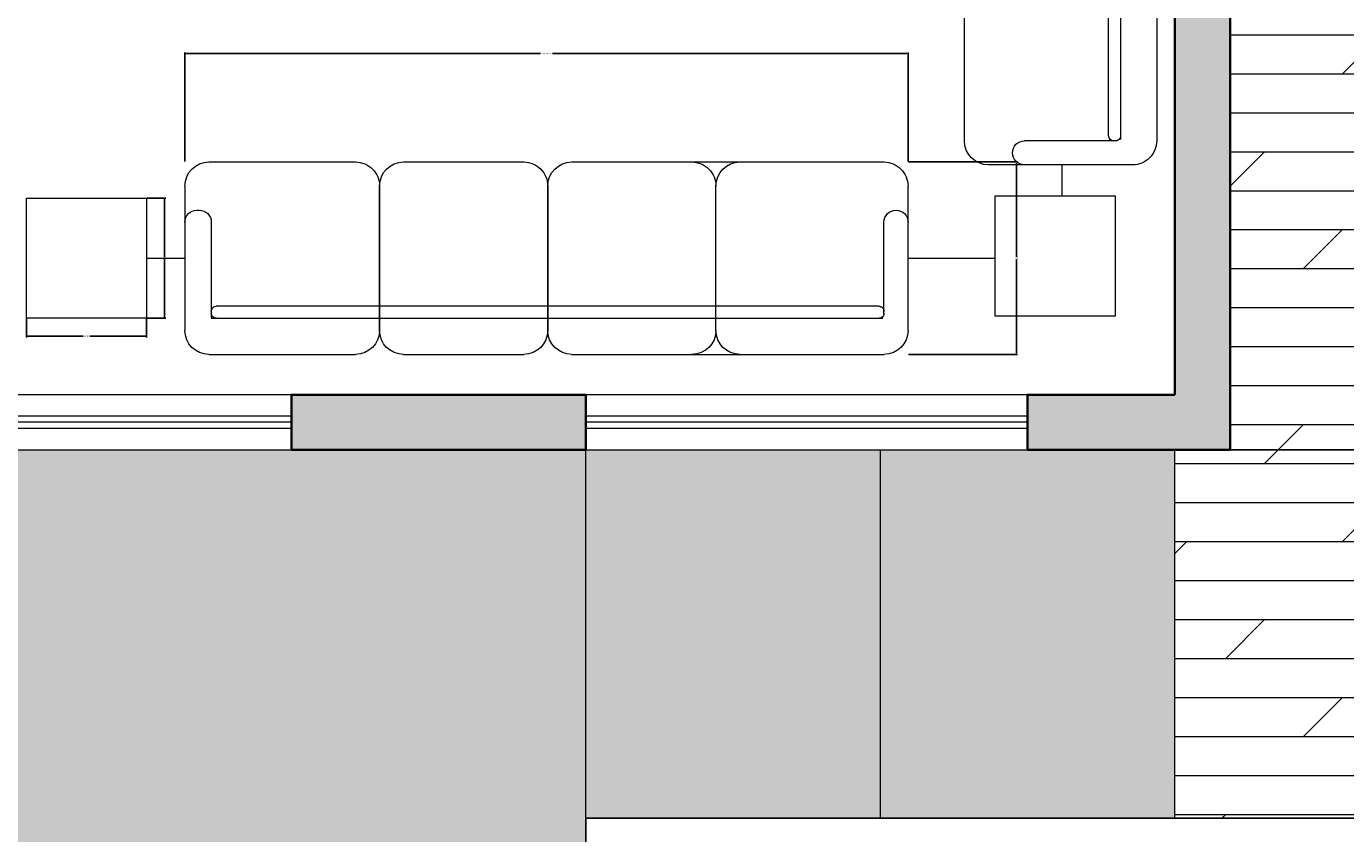
# Model space of a CAD drawing. Units: inches. Extents: x 84 to 1044, y -280 to 906.
# Tile 40 of 105: x 700 to 915, y 29 to 160. Entities that reach past the tile are written whole.
import ezdxf

# ---------------------------------------------------------------- set-up
doc = ezdxf.new("R2010")
doc.units = ezdxf.units.IN
for name, color, linetype, lineweight in [('A-ANNO-DIMS', 2, 'Continuous', 18), ('A-FURN', 8, 'Continuous', 15), ('L-HRDS', 32, 'Continuous', 18), ('L-POOL', 151, 'Continuous', 25), ('WALL', 250, 'Continuous', 35), ('WINDOW', 160, 'Continuous', 13)]:
    doc.layers.add(name, color=color, linetype=linetype, lineweight=lineweight)
for name, color, linetype, lineweight, true_color in [('A-FLOR-PATT', 251, 'Continuous', 9, 0x705861), ('A-WALL-PATT', 251, 'Continuous', 9, 0x636466), ('L-HRDS-PATT', 23, 'Continuous', 9, 0xc2877b), ('L-PLNT-PATT', 9, 'Continuous', 9, 0xafd9aa)]:
    doc.layers.add(name, color=color, linetype=linetype, lineweight=lineweight, true_color=true_color)
doc.styles.get("Standard").update_dxf_attribs({"font": 'arial.ttf'})
doc.dimstyles.get("Standard").update_dxf_attribs({"dimtxt": 0.18, "dimasz": 0.18, "dimexe": 0.18, "dimexo": 0.0625, "dimgap": 0.09, "dimtad": 0, "dimtih": 1, "dimtoh": 1, "dimdec": 4, "dimzin": 0, "dimdsep": 46, "dimtxsty": 'Standard', "dimcen": 0.09, "dimadec": 0, "dimazin": 0, "dimtfac": 1, "dimtdec": 4, "dimtofl": 0, "dimtmove": 0, "dimatfit": 3, "dimfxl": 1, "dimtolj": 1, "dimtzin": 0, "dimarcsym": 0})

# ---------------------------------------------------------------- blocks, each defined once
blk = doc.blocks.new('SOFA-4-SEAT')
for p, q in [((3.92, 31.33), (27.81, 31.33)), ((27.81, 31.33), (27.81, 31.33)), ((35.65, 31.33), (55.23, 31.33)), ((55.23, 31.33), (55.23, 31.33)), ((63.07, 31.33), (113.96, 31.33)), ((113.96, 31.33), (113.96, 31.33)), ((0, 3.91), (0, 27.42)), ((31.73, 27.42), (31.73, 3.91)), ((31.73, 3.91), (31.73, 27.42)), ((59.15, 3.91), (59.15, 27.42)), ((59.15, 27.42), (59.15, 3.91)), ((86.57, 27.42), (86.57, 3.91)), ((117.88, 27.42), (117.88, 3.91)), ((4.31, 12.82), (4.31, 25.46)), ((4.31, 25.46), (11.69, 25.46)), ((4.31, 24.28), (4.31, 24.67)), ((5.09, 25.46), (11.69, 25.46)), ((11.69, 25.46), (113.76, 25.46)), ((11.69, 25.46), (113.18, 25.46)), ((113.96, 24.67), (113.96, 24.28)), ((113.96, 24.28), (113.96, 9.79)), ((13.66, 23.5), (5.09, 23.5)), ((113.18, 23.5), (13.66, 23.5)), ((4.31, 9.79), (4.31, 12.82)), ((1.96, 7.83), (2.35, 7.83)), ((115.92, 7.83), (115.92, 7.83)), ((27.81, 0), (3.92, 0)), ((27.81, 0), (27.81, 0)), ((55.23, 0), (35.65, 0)), ((55.23, 0), (55.23, 0)), ((113.96, 0), (63.07, 0)), ((113.96, 0), (113.96, 0))]:
    blk.add_line(p, q)
for centre, radius, start, end in [((3.92, 27.42), 3.92, 90, 180), ((27.81, 27.42), 3.92, 0, 90), ((35.65, 27.42), 3.92, 90, 180), ((55.23, 27.42), 3.92, 0, 90), ((63.07, 27.42), 3.92, 90, 180), ((82.65, 27.42), 3.92, 0, 90), ((90.48, 27.42), 3.92, 90, 180), ((113.96, 27.42), 3.92, 0, 90), ((5.09, 24.67), 0.783, 90, 180), ((5.09, 24.28), 0.783, 180, 270), ((113.18, 24.67), 0.783, 0, 90), ((113.18, 24.28), 0.783, 270, 0), ((1.96, 9.79), 1.96, 180, 270), ((2.35, 9.79), 1.96, 270, 0), ((115.92, 9.79), 1.96, 180, 270), ((115.92, 9.79), 1.96, 270, 0), ((3.92, 3.91), 3.92, 180, 270), ((27.81, 3.91), 3.92, 270, 0), ((35.65, 3.91), 3.92, 180, 270), ((55.23, 3.91), 3.92, 270, 0), ((63.07, 3.91), 3.92, 180, 270), ((82.65, 3.91), 3.92, 270, 0), ((90.48, 3.91), 3.92, 180, 270), ((113.96, 3.91), 3.92, 270, 0)]:
    blk.add_arc(centre, radius, start, end)
blk = doc.blocks.new('SOFA-2-SEAT')
for p, q in [((27.42, 63.46), (3.92, 63.46)), ((7.83, 61.5), (7.83, 61.5)), ((0, 59.54), (0, 59.54)), ((0, 59.54), (0, 35.65)), ((24.29, 59.54), (9.79, 59.54)), ((23.5, 58.76), (23.5, 13.66)), ((24.68, 59.54), (24.29, 59.54)), ((25.46, 11.69), (25.46, 59.35)), ((25.46, 11.69), (25.46, 58.76)), ((31.34, 59.54), (31.34, 59.54)), ((31.34, 35.65), (31.34, 59.54)), ((3.92, 31.73), (27.42, 31.73)), ((27.42, 31.73), (3.92, 31.73)), ((0, 27.81), (0, 27.81)), ((0, 27.81), (0, 3.92)), ((31.34, 27.81), (31.34, 27.81)), ((31.34, 3.92), (31.34, 27.81)), ((23.5, 13.66), (23.5, 5.09)), ((25.46, 5.09), (25.46, 11.69)), ((25.46, 4.31), (25.46, 11.69)), ((9.79, 4.31), (12.83, 4.31)), ((12.83, 4.31), (25.46, 4.31)), ((24.29, 4.31), (24.68, 4.31)), ((7.83, 1.96), (7.83, 2.35)), ((3.92, 0), (27.42, 0))]:
    blk.add_line(p, q)
for centre, radius, start, end in [((3.92, 59.54), 3.92, 90, 180), ((9.79, 61.5), 1.96, 90, 180), ((27.42, 59.54), 3.92, 360, 90), ((9.79, 61.5), 1.96, 180, 270), ((24.29, 58.76), 0.783, 90, 180), ((24.68, 58.76), 0.783, 360, 90), ((3.92, 35.65), 3.92, 180, 270), ((27.42, 35.65), 3.92, 270, 360), ((3.92, 27.81), 3.92, 90, 180), ((27.42, 27.81), 3.92, 360, 90), ((9.79, 2.35), 1.96, 90, 180), ((24.29, 5.09), 0.783, 180, 270), ((24.68, 5.09), 0.783, 270, 360), ((3.92, 3.92), 3.92, 180, 270), ((27.42, 3.92), 3.92, 270, 360), ((9.79, 1.96), 1.96, 180, 270)]:
    blk.add_arc(centre, radius, start, end)
blk = doc.blocks.new('TABLE-END-SQUARE')
for p, q in [((0, 0), (0, 19.59)), ((0, 19.59), (19.58, 19.59)), ((19.58, 19.59), (19.58, 0)), ((19.58, 0), (0, 0))]:
    blk.add_line(p, q)
blk = doc.blocks.new('WIN-72IN')
for p, q in [((72, 9), (0, 9)), ((72, 5.5), (0, 5.5)), ((72, 4.5), (0, 4.5)), ((72, 3.5), (0, 3.5)), ((0, 0), (72, 0))]:
    blk.add_line(p, q)
blk = doc.blocks.new('*D52')
at = {"layer": 'A-ANNO-DIMS', "color": 0, "lineweight": -2, "transparency": 16777216}
for p, q in [((725.7, 138.09), (725.7, 155.89)), ((725.88, 155.71), (783.66, 155.71)), ((843.4, 155.71), (785.61, 155.71)), ((843.58, 138.09), (843.58, 155.89))]:
    blk.add_line(p, q, dxfattribs=at)
at = {"layer": 'A-ANNO-DIMS', "color": 0, "transparency": 16777216}
for points in [[(725.88, 155.74), (725.88, 155.68), (725.7, 155.71)], [(843.4, 155.74), (843.4, 155.68), (843.58, 155.71)]]:
    blk.add_solid(points, dxfattribs=at)
at = {"layer": 'Defpoints', "color": 0, "transparency": 16777216}
for p in [(843.58, 155.71), (725.7, 138.03), (843.58, 138.03)]:
    blk.add_point(p, dxfattribs=at)
at = {"layer": 'A-ANNO-DIMS', "color": 0, "transparency": 16777216, "insert": (784.64, 155.71), "char_height": 0.18, "attachment_point": 5}
blk.add_mtext('\\A1;SOFA 118 TYP.', dxfattribs=at)
blk = doc.blocks.new('*D53')
at = {"layer": 'A-ANNO-DIMS', "color": 0, "lineweight": -2, "transparency": 16777216}
for p, q in [((843.64, 138.03), (861.44, 138.03)), ((861.26, 137.85), (861.26, 122.54)), ((861.26, 106.87), (861.26, 122.18)), ((843.64, 106.69), (861.44, 106.69))]:
    blk.add_line(p, q, dxfattribs=at)
at = {"layer": 'A-ANNO-DIMS', "color": 0, "transparency": 16777216}
for points in [[(861.23, 137.85), (861.29, 137.85), (861.26, 138.03)], [(861.23, 106.87), (861.29, 106.87), (861.26, 106.69)]]:
    blk.add_solid(points, dxfattribs=at)
at = {"layer": 'Defpoints', "color": 0, "transparency": 16777216}
for p in [(843.58, 138.03), (843.58, 106.69), (861.26, 106.69)]:
    blk.add_point(p, dxfattribs=at)
at = {"layer": 'A-ANNO-DIMS', "color": 0, "transparency": 16777216, "insert": (861.26, 122.36), "char_height": 0.18, "attachment_point": 5}
blk.add_mtext('\\A1;31 TYP.', dxfattribs=at)
blk = doc.blocks.new('*D56')
at = {"layer": 'A-ANNO-DIMS', "color": 0, "lineweight": -2, "transparency": 16777216}
for p, q in [((719.51, 132.15), (722.57, 132.15)), ((722.39, 131.97), (722.39, 122.54)), ((722.39, 112.75), (722.39, 122.18)), ((719.51, 112.57), (722.57, 112.57))]:
    blk.add_line(p, q, dxfattribs=at)
at = {"layer": 'A-ANNO-DIMS', "color": 0, "transparency": 16777216}
for points in [[(722.36, 131.97), (722.42, 131.97), (722.39, 132.15)], [(722.36, 112.75), (722.42, 112.75), (722.39, 112.57)]]:
    blk.add_solid(points, dxfattribs=at)
at = {"layer": 'Defpoints', "color": 0, "transparency": 16777216}
for p in [(719.45, 132.15), (722.39, 132.15), (719.45, 112.57)]:
    blk.add_point(p, dxfattribs=at)
at = {"layer": 'A-ANNO-DIMS', "color": 0, "transparency": 16777216, "insert": (722.39, 122.36), "char_height": 0.18, "attachment_point": 5}
blk.add_mtext('\\A1;END TABLE 20 TYP.', dxfattribs=at)
blk = doc.blocks.new('*D57')
at = {"layer": 'A-ANNO-DIMS', "color": 0, "lineweight": -2, "transparency": 16777216}
for p, q in [((699.86, 112.5), (699.86, 109.45)), ((719.45, 112.5), (719.45, 109.45)), ((700.04, 109.63), (709.13, 109.63)), ((719.27, 109.63), (710.19, 109.63))]:
    blk.add_line(p, q, dxfattribs=at)
at = {"layer": 'A-ANNO-DIMS', "color": 0, "transparency": 16777216}
for points in [[(700.04, 109.66), (700.04, 109.6), (699.86, 109.63)], [(719.27, 109.66), (719.27, 109.6), (719.45, 109.63)]]:
    blk.add_solid(points, dxfattribs=at)
at = {"layer": 'Defpoints', "color": 0, "transparency": 16777216}
for p in [(699.86, 112.57), (719.45, 112.57), (719.45, 109.63)]:
    blk.add_point(p, dxfattribs=at)
at = {"layer": 'A-ANNO-DIMS', "color": 0, "transparency": 16777216, "insert": (709.66, 109.63), "char_height": 0.18, "attachment_point": 5}
blk.add_mtext('\\A1;20 TYP.', dxfattribs=at)
blk = doc.blocks.new('*D63')
at = {"layer": 'A-ANNO-DIMS', "color": 0, "lineweight": -2, "transparency": 16777216}
for p, q in [((833.14, 709.12), (1043.77, 709.12)), ((1043.59, 708.94), (1043.59, 400.3)), ((1043.59, 91.3), (1043.59, 399.94)), ((896.14, 91.12), (1043.77, 91.12))]:
    blk.add_line(p, q, dxfattribs=at)
at = {"layer": 'A-ANNO-DIMS', "color": 0, "transparency": 16777216}
for points in [[(1043.56, 708.94), (1043.62, 708.94), (1043.59, 709.12)], [(1043.56, 91.3), (1043.62, 91.3), (1043.59, 91.12)]]:
    blk.add_solid(points, dxfattribs=at)
at = {"layer": 'Defpoints', "color": 0, "transparency": 16777216}
for p in [(833.07, 709.12), (1043.59, 709.12), (896.07, 91.12)]:
    blk.add_point(p, dxfattribs=at)
at = {"layer": 'A-ANNO-DIMS', "color": 0, "transparency": 16777216, "insert": (1043.59, 400.12), "char_height": 0.18, "attachment_point": 5}
blk.add_mtext('\\A1;618', dxfattribs=at)
blk = doc.blocks.new('*D69')
at = {"layer": 'A-ANNO-DIMS', "color": 0, "lineweight": -2, "transparency": 16777216}
for p, q in [((896.14, 91.12), (1043.77, 91.12)), ((1043.59, 90.94), (1043.59, 61.3)), ((1043.59, 31.3), (1043.59, 60.94)), ((983.14, 31.12), (1043.77, 31.12))]:
    blk.add_line(p, q, dxfattribs=at)
at = {"layer": 'A-ANNO-DIMS', "color": 0, "transparency": 16777216}
for points in [[(1043.56, 90.94), (1043.62, 90.94), (1043.59, 91.12)], [(1043.56, 31.3), (1043.62, 31.3), (1043.59, 31.12)]]:
    blk.add_solid(points, dxfattribs=at)
at = {"layer": 'Defpoints', "color": 0, "transparency": 16777216}
for p in [(896.07, 91.12), (983.07, 31.12), (1043.59, 31.12)]:
    blk.add_point(p, dxfattribs=at)
at = {"layer": 'A-ANNO-DIMS', "color": 0, "transparency": 16777216, "insert": (1043.59, 61.12), "char_height": 0.18, "attachment_point": 5}
blk.add_mtext('\\A1;60', dxfattribs=at)

msp = doc.modelspace()

# ---------------------------------------------------------------- hatches: boundary and pattern name
at = {"layer": 'A-FLOR-PATT', "transparency": 33554597}
h = msp.add_hatch(dxfattribs=at)
h.set_pattern_fill('DOLMIT', color=256)
h.paths.add_polyline_path([(983.074, 265.12), (896.074, 265.12), (896.074, 91.12), (887.074, 91.12), (887.074, 31.12), (983.074, 31.12)])
at = {"layer": 'A-WALL-PATT', "transparency": 33554597}
h = msp.add_hatch(color=256, dxfattribs=at)
h.dxf.hatch_style = 1
h.paths.add_polyline_path([(671.074, 100.12), (647.074, 100.12), (647.074, 160.12), (641.074, 160.12), (620.824, 160.12), (620.824, 151.12), (638.074, 151.12), (638.074, 91.12), (671.074, 91.12)])
h.paths.add_polyline_path([(791.074, 100.12), (743.074, 100.12), (743.074, 91.12), (791.074, 91.12)])
h.paths.add_polyline_path([(896.074, 346.12), (887.074, 346.12), (887.074, 334.12), (870.955, 334.12), (833.074, 334.12), (804.574, 334.12), (804.574, 328.12), (887.074, 328.12), (887.074, 100.12), (863.074, 100.12), (863.074, 91.12), (896.074, 91.12)])
h.paths.add_polyline_path([(507.574, 154.729), (507.574, 160.12), (464.074, 160.12), (464.074, 247.12), (641.074, 247.12), (641.074, 208.12), (647.074, 208.12), (647.074, 328.12), (659.074, 328.12), (659.074, 334.12), (617.074, 334.12), (617.074, 328.12), (641.074, 328.12), (641.074, 256.12), (545.074, 256.12), (545.074, 328.12), (569.074, 328.12), (569.074, 334.12), (518.074, 334.12), (518.074, 325.12), (536.074, 325.12), (536.074, 256.12), (464.074, 256.12), (464.074, 325.12), (482.074, 325.12), (482.074, 334.12), (455.074, 334.12), (455.074, 160.12), (413.127, 160.12), (413.127, 151.12), (455.074, 151.12), (455.074, 91.12), (464.074, 91.12), (464.074, 151.12), (507.574, 151.12)])
h.paths.add_polyline_path([(572.824, 160.12), (555.574, 160.12), (555.574, 151.12), (572.824, 151.12)], flags=17)
h.paths.add_polyline_path([(341.127, 160.12), (299.179, 160.12), (299.179, 211.12), (294.179, 211.12), (290.179, 211.12), (290.179, 151.12), (341.127, 151.12)])
h.paths.add_polyline_path([(299.179, 256.12), (212.179, 256.12), (212.179, 274.12), (203.179, 274.12), (203.179, 247.12), (299.179, 247.12)])
h.paths.add_polyline_path([(212.179, 514.12), (398.074, 514.12), (398.074, 519.12), (398.074, 520.12), (212.179, 520.12), (212.179, 574.12), (203.179, 574.12), (203.179, 310.12), (212.179, 310.12), (212.179, 328.12), (290.179, 328.12), (290.179, 292.12), (299.179, 292.12), (299.179, 328.12), (332.179, 328.12), (332.179, 334.12), (212.179, 334.12)])
h.paths.add_polyline_path([(287.127, 709.12), (203.179, 709.12), (203.179, 646.12), (212.179, 646.12), (212.179, 700.12), (287.127, 700.12)])
h.paths.add_polyline_path([(470.074, 709.12), (359.127, 709.12), (359.127, 700.12), (434.074, 700.12), (434.074, 574.12), (440.074, 574.12), (440.074, 622.12), (464.074, 622.12), (464.074, 628.12), (440.074, 628.12), (440.074, 700.12), (470.074, 700.12)])
h.paths.add_polyline_path([(572.074, 709.12), (506.074, 709.12), (506.074, 700.12), (536.074, 700.12), (536.074, 628.12), (494.074, 628.12), (494.074, 622.12), (536.074, 622.12), (536.074, 520.12), (440.074, 520.12), (440.074, 544.12), (434.074, 544.12), (434.074, 514.12), (644.074, 514.12), (644.074, 519.12), (644.074, 544.12), (638.074, 544.12), (638.074, 520.12), (542.074, 520.12), (542.074, 622.12), (584.074, 622.12), (584.074, 628.12), (542.074, 628.12), (542.074, 700.12), (572.074, 700.12)])
h.paths.add_polyline_path([(698.074, 709.12), (608.074, 709.12), (608.074, 700.12), (638.074, 700.12), (638.074, 628.12), (614.074, 628.12), (614.074, 622.12), (638.074, 622.12), (638.074, 574.12), (644.074, 574.12), (644.074, 700.12), (698.074, 700.12)])
h.paths.add_polyline_path([(833.074, 709.12), (770.074, 709.12), (770.074, 700.12), (824.074, 700.12), (824.074, 646.12), (833.074, 646.12)])
h.paths.add_polyline_path([(833.074, 574.12), (824.074, 574.12), (824.074, 520.12), (791.244, 520.12), (712.904, 520.12), (680.074, 520.12), (680.074, 514.12), (695.074, 514.12), (695.074, 491.62), (704.074, 491.62), (704.074, 511.12), (833.074, 511.12)])
h.paths.add_polyline_path([(704.074, 419.62), (695.074, 419.62), (695.074, 370.12), (704.074, 370.12)])
h.paths.add_polyline_path([(896.074, 400.12), (833.074, 400.12), (833.074, 364.12), (839.074, 364.12), (839.074, 394.12), (887.074, 394.12), (887.074, 382.12), (896.074, 382.12)])
h.paths.add_polyline_path([(732.574, 334.12), (695.074, 334.12), (695.074, 328.12), (732.574, 328.12)])
at = {"layer": 'L-HRDS-PATT', "transparency": 33554597}
h = msp.add_hatch(color=256, dxfattribs=at)
h.dxf.hatch_style = 1
h.paths.add_polyline_path([(839.074, 91.12), (791.074, 91.12), (791.074, 31.12), (839.074, 31.12)])
h.paths.add_polyline_path([(887.074, 91.12), (863.074, 91.12), (839.074, 91.12), (839.074, 31.12), (887.074, 31.12)])
at = {"layer": 'L-PLNT-PATT', "transparency": 33554597}
h = msp.add_hatch(color=256, dxfattribs=at)
h.dxf.hatch_style = 1
h.paths.add_polyline_path([(791.074, 31.12), (791.074, 91.12), (743.074, 91.12), (674.074, 91.12), (674.074, 31.12), (650.074, 31.12), (650.074, -112.88), (983.074, -112.88), (983.074, -64.88), (791.074, -64.88)])

# ---------------------------------------------------------------- linework, layer by layer
at = {"layer": 'A-FURN'}
for p, q in [((868.727, 132.507), (868.727, 137.568)), ((719.448, 122.358), (725.702, 122.358)), ((843.576, 122.358), (857.76, 122.358)), ((789.915, 106.694), (789.915, 106.694))]:
    msp.add_line(p, q, dxfattribs=at)
at = {"layer": 'L-HRDS'}
for p, q in [((791.074, 31.12), (791.074, 91.12)), ((839.074, 31.12), (839.074, 91.12)), ((887.074, 31.12), (887.074, 91.12))]:
    msp.add_line(p, q, dxfattribs=at)
at = {"layer": 'L-POOL'}
msp.add_lwpolyline([(791.074, 31.12), (983.074, 31.12), (983.074, -64.88), (791.074, -64.88)], close=True, dxfattribs=at)
at = {"layer": 'WALL'}
for p, q in [((896.074, 91.12), (896.074, 346.12)), ((887.074, 100.12), (887.074, 328.12)), ((743.074, 100.12), (743.074, 91.12)), ((743.074, 100.12), (791.074, 100.12)), ((791.074, 91.12), (791.074, 100.12)), ((863.074, 91.12), (863.074, 100.12)), ((863.074, 100.12), (887.074, 100.12)), ((743.074, 91.12), (791.074, 91.12)), ((863.074, 91.12), (896.074, 91.12))]:
    msp.add_line(p, q, dxfattribs=at)

# ---------------------------------------------------------------- block references
at = {"layer": 'A-FURN', "extrusion": (0, 0, -1), "zscale": -1, "rotation": 180}
for name, p in [('SOFA-2-SEAT', (-852.77, 201.026)), ('SOFA-4-SEAT', (-725.7, 138.023))]:
    msp.add_blockref(name, p, dxfattribs=at)
at = {"layer": 'A-FURN'}
for p in [(699.864, 112.563), (857.76, 112.919)]:
    msp.add_blockref('TABLE-END-SQUARE', p, dxfattribs=at)
at = {"layer": 'WINDOW'}
for p in [(671.07, 91.12), (791.07, 91.12)]:
    msp.add_blockref('WIN-72IN', p, dxfattribs=at)

# ---------------------------------------------------------------- dimensions: what is measured, and where the dimension line sits
at = {"layer": 'A-ANNO-DIMS'}
for base, p2, picture, middle in [((1043.588, 709.12), (833.074, 709.12), '*D63', (1043.588, 400.12)), ((1043.588, 31.12), (983.074, 31.12), '*D69', (1043.588, 61.12))]:
    dim = msp.add_linear_dim(base=base, p1=(896.074, 91.12), p2=p2, angle=90, dimstyle='Standard', override={"dimdec": 0, "dimlfac": 1, "dimrnd": 0, "dimzin": 0, "dimdsep": 46, "dimlunit": 2}, dxfattribs=at)
    dim.commit()
    dim.dimension.update_dxf_attribs({"geometry": picture, "text_midpoint": middle})
for base, p1, p2, angle, text, picture, middle in [((843.576, 155.707), (725.702, 138.026), (843.576, 138.026), 0, 'SOFA <> TYP.', '*D52', (784.639, 155.707)), ((861.257, 106.69), (843.576, 138.026), (843.576, 106.69), 270, '<> TYP.', '*D53', (861.257, 122.358)), ((722.386, 132.15), (719.448, 112.565), (719.448, 132.15), 90, 'END TABLE <> TYP.', '*D56', (722.386, 122.358))]:
    dim = msp.add_linear_dim(base=base, p1=p1, p2=p2, angle=angle, text=text, dimstyle='Standard', override={"dimdec": 0, "dimlfac": 1, "dimrnd": 0, "dimzin": 0, "dimdsep": 46, "dimlunit": 2}, dxfattribs=at)
    dim.commit()
    dim.dimension.update_dxf_attribs({"geometry": picture, "text_midpoint": middle})
dim = msp.add_linear_dim(base=(719.448, 109.627), p1=(699.863, 112.565), p2=(719.448, 112.565), text='<> TYP.', dimstyle='Standard', override={"dimdec": 0, "dimlfac": 1, "dimrnd": 0, "dimzin": 0, "dimdsep": 46, "dimlunit": 2}, dxfattribs=at)
dim.commit()
dim.dimension.update_dxf_attribs({"geometry": '*D57', "text_midpoint": (709.656, 109.627)})

doc.saveas('drawing.dxf')
